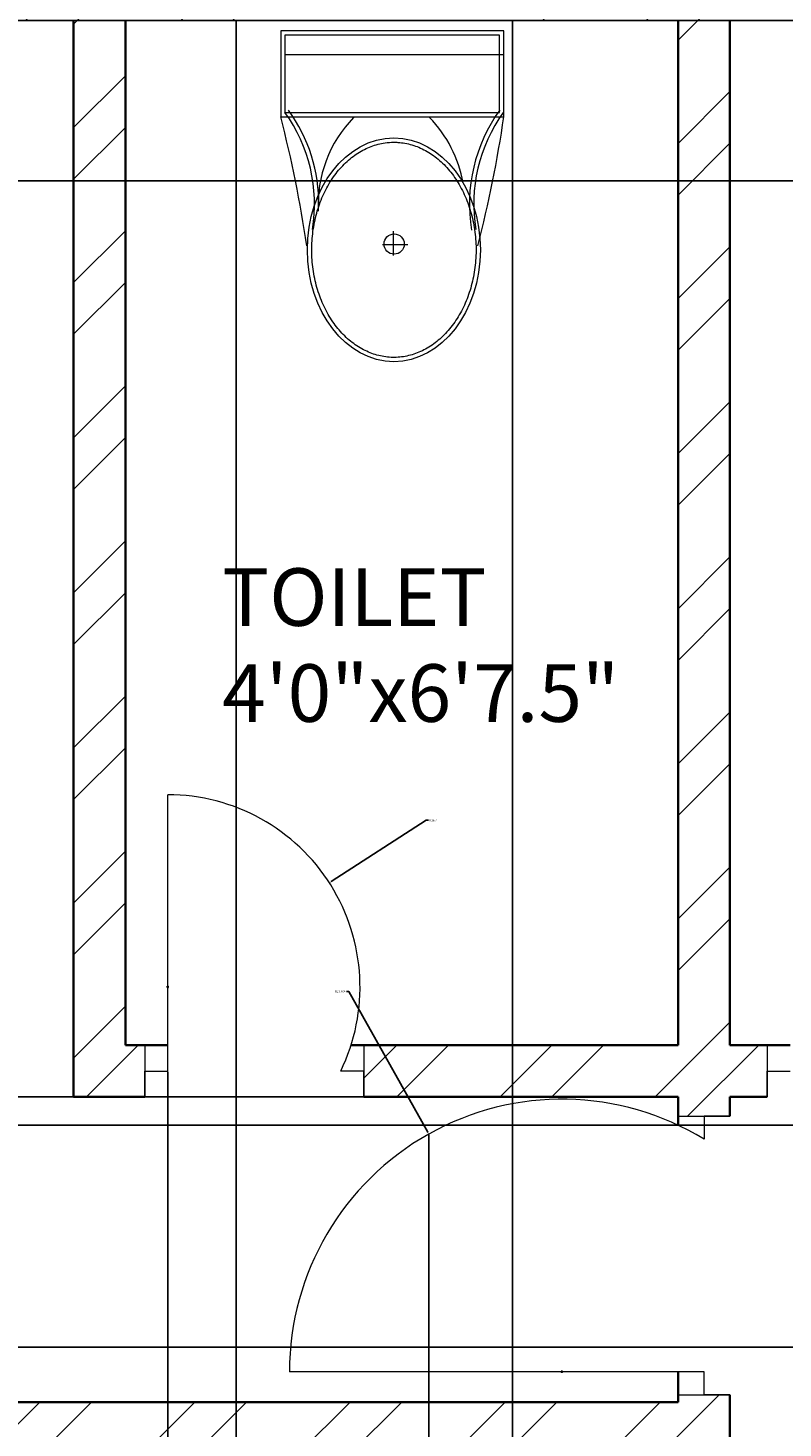
# Model space of a CAD drawing. Units: inches. Extents: x 1748 to 2382, y 1346 to 2284.
# Tile 23 of 26: x 2022 to 2088, y 2102 to 2223. Entities that reach past the tile are written whole.
import ezdxf

# ---------------------------------------------------------------- set-up
doc = ezdxf.new("R2010")
doc.units = ezdxf.units.IN
for name, color, linetype, lineweight in [('A-ANNO-DIMS', 2, 'Continuous', 18), ('A-AREA-IDEN', 7, 'Continuous', 18), ('A-DOOR', 21, 'Continuous', 18), ('A-FLOR-FIXT', 7, 'Continuous', 18), ('A-WALL', 7, 'Continuous', 35), ('A-WALL-PATT', 9, 'Continuous', 13)]:
    doc.layers.add(name, color=color, linetype=linetype, lineweight=lineweight)
doc.styles.get("Standard").update_dxf_attribs({"font": 'arial.ttf'})
doc.dimstyles.get("Standard").update_dxf_attribs({"dimtxt": 0.18, "dimasz": 0.18, "dimexe": 0.18, "dimexo": 0.0625, "dimgap": 0.09, "dimtad": 0, "dimtih": 1, "dimtoh": 1, "dimdec": 4, "dimzin": 0, "dimdsep": 46, "dimtxsty": 'Standard', "dimcen": 0.09, "dimadec": 0, "dimazin": 0, "dimtfac": 1, "dimtdec": 4, "dimtofl": 0, "dimtmove": 0, "dimatfit": 3, "dimfxl": 1, "dimtolj": 1, "dimtzin": 0, "dimarcsym": 0})

# ---------------------------------------------------------------- blocks, each defined once
blk = doc.blocks.new('A$C31115884')
for p, q in [((257.5, 466.4), (257.5, 523.2)), ((283.1, 497.7), (223.4, 497.7)), ((0, 200), (0, 0)), ((520, 200), (0, 200)), ((520, 0), (520, 200)), ((10, 190), (10, 10)), ((510, 190), (10, 190)), ((510, 10), (510, 190)), ((510, 54.5), (0, 54.5)), ((10, 10), (510, 10)), ((0, 0), (520, 0))]:
    blk.add_line(p, q)
blk.add_circle((255.6, 496.4), 23.6)
for centre, radius, start, end in [((2777.7, -204.6), 2807, 165.4549, 171.7133), ((3237, 905), 2807, 188.2867, 194.5451), ((-294.5, 403.3), 364.7, 324.2091, 9.3499), ((-294.5, 403.3), 374.7, 324.2091, 9.3499), ((805.8, 403.3), 364.7, 170.6501, 215.7909), ((139.5, 406.2), 293.5, 315.8436, 2.6563), ((805.8, 403.3), 374.7, 179.2036, 215.7909), ((383.6, 406.2), 293.5, 190.2774, 224.1564)]:
    blk.add_arc(centre, radius, start, end)
blk.add_ellipse((256.2, 509.9), major_axis=(0, -260.7), ratio=0.772727)
blk.add_open_spline([(256.2, 259.2), (263.1, 259.2), (270, 259.7), (287.8, 262.3), (298.7, 265.1), (319.9, 273.1), (330.2, 278.4), (350.1, 291.1), (359.7, 298.7), (377.7, 315.9), (386.2, 325.5), (401.7, 346.6), (408.8, 358.1), (421.3, 382.5), (426.8, 395.5), (435.9, 422.4), (439.5, 436.4), (444.8, 465.1), (446.5, 479.7), (447.9, 509.2), (447.6, 524), (445, 553.3), (442.7, 567.8), (436.3, 596), (432.1, 609.7), (421.9, 636), (416, 648.6), (402.5, 672.1), (395, 683), (378.6, 703), (369.8, 712.1), (351.1, 728), (341.3, 734.8), (320.9, 746.2), (310.4, 750.7), (288.9, 757.3), (278, 759.4), (256, 761), (245, 760.6), (223.1, 757.2), (212.3, 754.3), (191.1, 746.1), (180.8, 740.7), (160.9, 727.8), (151.4, 720.1), (133.5, 702.7), (125.1, 693), (109.6, 671.7), (102.6, 660.2), (90.2, 635.7), (84.9, 622.7), (76, 595.6), (72.4, 581.6), (67.2, 552.9), (65.6, 538.2), (64.4, 508.8), (64.8, 494), (67.5, 464.7), (69.9, 450.2), (76.6, 422), (80.8, 408.3), (91.1, 382.2), (97.2, 369.7), (110.8, 346.3), (118.4, 335.4), (134.8, 315.6), (143.7, 306.7), (162.4, 290.9), (172.3, 284.2), (192.8, 273), (203.3, 268.6), (224.8, 262.2), (235.8, 260.2), (249.9, 259.3), (253, 259.2), (256.2, 259.2)], degree=3, knots=[0, 0, 0, 0, 0.110105, 0.110105, 0.285049, 0.285049, 0.459994, 0.459994, 0.634938, 0.634938, 0.809882, 0.809882, 0.984827, 0.984827, 1.159771, 1.159771, 1.334715, 1.334715, 1.50966, 1.50966, 1.684604, 1.684604, 1.859549, 1.859549, 2.034493, 2.034493, 2.209437, 2.209437, 2.384382, 2.384382, 2.559326, 2.559326, 2.73427, 2.73427, 2.909215, 2.909215, 3.084159, 3.084159, 3.259103, 3.259103, 3.434048, 3.434048, 3.608992, 3.608992, 3.783936, 3.783936, 3.958881, 3.958881, 4.133825, 4.133825, 4.30877, 4.30877, 4.483714, 4.483714, 4.658658, 4.658658, 4.833603, 4.833603, 5.008547, 5.008547, 5.183491, 5.183491, 5.358436, 5.358436, 5.53338, 5.53338, 5.708324, 5.708324, 5.883269, 5.883269, 6.058213, 6.058213, 6.233158, 6.233158, 6.283185, 6.283185, 6.283185, 6.283185])
blk = doc.blocks.new('*D51')
at = {"layer": 'A-ANNO-DIMS', "color": 0, "lineweight": -2, "transparency": 16777216}
for p, q in [((1968.44, 2223.79), (1968.44, 1360.47)), ((2040.07, 2223.79), (2040.07, 1360.47)), ((1968.62, 1360.65), (2003.86, 1360.65)), ((2039.89, 1360.65), (2004.65, 1360.65))]:
    blk.add_line(p, q, dxfattribs=at)
at = {"layer": 'A-ANNO-DIMS', "color": 0, "transparency": 16777216}
for points in [[(1968.62, 1360.68), (1968.62, 1360.62), (1968.44, 1360.65)], [(2039.89, 1360.68), (2039.89, 1360.62), (2040.07, 1360.65)]]:
    blk.add_solid(points, dxfattribs=at)
at = {"layer": 'Defpoints', "color": 0, "transparency": 16777216}
for p in [(1968.44, 2223.85), (2040.07, 2223.85), (2040.07, 1360.65)]:
    blk.add_point(p, dxfattribs=at)
at = {"layer": 'A-ANNO-DIMS', "color": 0, "transparency": 16777216, "insert": (2004.26, 1360.65), "char_height": 0.18, "attachment_point": 5}
blk.add_mtext('\\A1;71.62', dxfattribs=at)
blk = doc.blocks.new('*D52')
at = {"layer": 'A-ANNO-DIMS', "color": 0, "lineweight": -2, "transparency": 16777216}
for p, q in [((2064.07, 2223.79), (2064.07, 1360.47)), ((2091.4, 2223.79), (2091.4, 1360.47)), ((2064.25, 1360.65), (2077.34, 1360.65)), ((2091.22, 1360.65), (2078.13, 1360.65))]:
    blk.add_line(p, q, dxfattribs=at)
at = {"layer": 'A-ANNO-DIMS', "color": 0, "transparency": 16777216}
for points in [[(2064.25, 1360.68), (2064.25, 1360.62), (2064.07, 1360.65)], [(2091.22, 1360.68), (2091.22, 1360.62), (2091.4, 1360.65)]]:
    blk.add_solid(points, dxfattribs=at)
at = {"layer": 'Defpoints', "color": 0, "transparency": 16777216}
for p in [(2064.07, 2223.85), (2091.4, 2223.85), (2091.4, 1360.65)]:
    blk.add_point(p, dxfattribs=at)
at = {"layer": 'A-ANNO-DIMS', "color": 0, "transparency": 16777216, "insert": (2077.73, 1360.65), "char_height": 0.18, "attachment_point": 5}
blk.add_mtext('\\A1;27.33', dxfattribs=at)
blk = doc.blocks.new('*D68')
at = {"layer": 'A-ANNO-DIMS', "color": 0, "lineweight": -2, "transparency": 16777216}
for p, q in [((1865.52, 2223.85), (2339.54, 2223.85)), ((2339.36, 2223.67), (2339.36, 2217.07)), ((2339.36, 2210.1), (2339.36, 2216.7)), ((1865.52, 2209.92), (2339.54, 2209.92))]:
    blk.add_line(p, q, dxfattribs=at)
at = {"layer": 'A-ANNO-DIMS', "color": 0, "transparency": 16777216}
for points in [[(2339.33, 2223.67), (2339.39, 2223.67), (2339.36, 2223.85)], [(2339.33, 2210.1), (2339.39, 2210.1), (2339.36, 2209.92)]]:
    blk.add_solid(points, dxfattribs=at)
at = {"layer": 'Defpoints', "color": 0, "transparency": 16777216}
for p in [(1865.46, 2223.85), (2339.36, 2223.85), (1865.46, 2209.92)]:
    blk.add_point(p, dxfattribs=at)
at = {"layer": 'A-ANNO-DIMS', "color": 0, "transparency": 16777216, "insert": (2339.36, 2216.88), "char_height": 0.18, "attachment_point": 5}
blk.add_mtext('\\A1;13.93', dxfattribs=at)
blk = doc.blocks.new('*D75')
at = {"layer": 'A-ANNO-DIMS', "color": 0, "lineweight": -2, "transparency": 16777216}
for p, q in [((2078.4, 2130.35), (1779.88, 2130.35)), ((1780.06, 2130.17), (1780.06, 2117.28)), ((1780.06, 2104.03), (1780.06, 2116.92)), ((2078.4, 2103.85), (1779.88, 2103.85))]:
    blk.add_line(p, q, dxfattribs=at)
at = {"layer": 'A-ANNO-DIMS', "color": 0, "transparency": 16777216}
for points in [[(1780.03, 2130.17), (1780.09, 2130.17), (1780.06, 2130.35)], [(1780.03, 2104.03), (1780.09, 2104.03), (1780.06, 2103.85)]]:
    blk.add_solid(points, dxfattribs=at)
at = {"layer": 'Defpoints', "color": 0, "transparency": 16777216}
for p in [(1780.06, 2130.35), (2078.46, 2130.35), (2078.46, 2103.85)]:
    blk.add_point(p, dxfattribs=at)
at = {"layer": 'A-ANNO-DIMS', "color": 0, "transparency": 16777216, "insert": (1780.06, 2117.1), "char_height": 0.18, "attachment_point": 5}
blk.add_mtext('\\A1;26.5', dxfattribs=at)
blk = doc.blocks.new('*D77')
at = {"layer": 'A-ANNO-DIMS', "color": 0, "lineweight": -2, "transparency": 16777216}
for p, q in [((1870.02, 2127.89), (2339.54, 2127.89)), ((2339.36, 2127.71), (2339.36, 2118.43)), ((2339.36, 2108.79), (2339.36, 2118.07)), ((1870.02, 2108.61), (2339.54, 2108.61))]:
    blk.add_line(p, q, dxfattribs=at)
at = {"layer": 'A-ANNO-DIMS', "color": 0, "transparency": 16777216}
for points in [[(2339.33, 2127.71), (2339.39, 2127.71), (2339.36, 2127.89)], [(2339.33, 2108.79), (2339.39, 2108.79), (2339.36, 2108.61)]]:
    blk.add_solid(points, dxfattribs=at)
at = {"layer": 'Defpoints', "color": 0, "transparency": 16777216}
for p in [(1869.96, 2127.89), (2339.36, 2127.89), (1869.96, 2108.61)]:
    blk.add_point(p, dxfattribs=at)
at = {"layer": 'A-ANNO-DIMS', "color": 0, "transparency": 16777216, "insert": (2339.36, 2118.25), "char_height": 0.18, "attachment_point": 5}
blk.add_mtext('\\A1;19.288', dxfattribs=at)
blk = doc.blocks.new('*D78')
at = {"layer": 'A-ANNO-DIMS', "color": 0, "lineweight": -2, "transparency": 16777216}
for p, q in [((2034.13, 2132.54), (2034.13, 1360.47)), ((2056.8, 2127.06), (2056.8, 1360.47)), ((2034.31, 1360.65), (2045, 1360.65)), ((2056.62, 1360.65), (2045.93, 1360.65))]:
    blk.add_line(p, q, dxfattribs=at)
at = {"layer": 'A-ANNO-DIMS', "color": 0, "transparency": 16777216}
for points in [[(2034.31, 1360.68), (2034.31, 1360.62), (2034.13, 1360.65)], [(2056.62, 1360.68), (2056.62, 1360.62), (2056.8, 1360.65)]]:
    blk.add_solid(points, dxfattribs=at)
at = {"layer": 'Defpoints', "color": 0, "transparency": 16777216}
for p in [(2034.13, 2132.6), (2056.8, 2127.13), (2056.8, 1360.65)]:
    blk.add_point(p, dxfattribs=at)
at = {"layer": 'A-ANNO-DIMS', "color": 0, "transparency": 16777216, "insert": (2045.47, 1360.65), "char_height": 0.18, "attachment_point": 5}
blk.add_mtext('\\A1;22.663', dxfattribs=at)
blk = doc.blocks.new('*D88')
at = {"layer": 'A-ANNO-DIMS', "color": 0, "lineweight": -2, "transparency": 16777216}
for p, q in [((2049.67, 2139.51), (2049.85, 2139.51)), ((2049.85, 2139.51), (2056.71, 2127.28)), ((2068.28, 2106.49), (2068.46, 2106.49)), ((2068.37, 2106.4), (2068.37, 2106.58))]:
    blk.add_line(p, q, dxfattribs=at)
at = {"layer": 'A-ANNO-DIMS', "color": 0, "transparency": 16777216}
blk.add_solid([(2056.74, 2127.3), (2056.68, 2127.27), (2056.8, 2127.13)], dxfattribs=at)
at = {"layer": 'Defpoints', "color": 0, "transparency": 16777216}
for p in [(2056.8, 2127.13), (2068.37, 2106.49)]:
    blk.add_point(p, dxfattribs=at)
at = {"layer": 'A-ANNO-DIMS', "color": 0, "transparency": 16777216, "insert": (2049.12, 2139.51), "char_height": 0.18, "attachment_point": 5}
blk.add_mtext('\\A1;R23.664', dxfattribs=at)
blk = doc.blocks.new('*D99')
at = {"layer": 'A-ANNO-DIMS', "color": 0, "lineweight": -2, "transparency": 16777216}
for p, q in [((2056.59, 2154.38), (2048.32, 2149.05)), ((2056.77, 2154.38), (2056.59, 2154.38)), ((2034.13, 2139.81), (2034.13, 2139.99)), ((2034.04, 2139.9), (2034.22, 2139.9))]:
    blk.add_line(p, q, dxfattribs=at)
at = {"layer": 'A-ANNO-DIMS', "color": 0, "transparency": 16777216}
blk.add_solid([(2048.31, 2149.07), (2048.34, 2149.02), (2048.17, 2148.95)], dxfattribs=at)
at = {"layer": 'Defpoints', "color": 0, "transparency": 16777216}
for p in [(2048.17, 2148.95), (2034.13, 2139.9)]:
    blk.add_point(p, dxfattribs=at)
at = {"layer": 'A-ANNO-DIMS', "color": 0, "transparency": 16777216, "insert": (2057.18, 2154.38), "char_height": 0.18, "attachment_point": 5}
blk.add_mtext('\\A1;R16.7', dxfattribs=at)

msp = doc.modelspace()

# ---------------------------------------------------------------- hatches: boundary and pattern name
at = {"layer": 'A-WALL-PATT'}
h = msp.add_hatch(dxfattribs=at)
h.set_pattern_fill('ANSI32', color=256)
h.paths.add_polyline_path([(1908.4445, 2232.8497), (1821.9607, 2232.8497), (1821.9607, 2223.8497), (1865.4607, 2223.8497), (1865.4607, 2209.9185), (1869.9607, 2209.9185), (1869.9607, 2223.8497), (1908.4445, 2223.8497), (1908.4445, 2228.3497)])
h.paths.add_polyline_path([(2040.0683, 2232.8497), (1968.4445, 2232.8497), (1968.4445, 2223.8497), (2025.9607, 2223.8497), (2025.9607, 2130.3497), (2032.1341, 2130.3497), (2032.1341, 2132.5997), (2032.1341, 2134.8497), (2030.4607, 2134.8497), (2030.4607, 2223.8497), (2040.0683, 2223.8497)])
h.paths.add_polyline_path([(2091.3969, 2232.8497), (2064.0683, 2232.8497), (2064.0683, 2223.8497), (2078.4607, 2223.8497), (2078.4607, 2134.8497), (2051.1563, 2134.8497), (2051.1563, 2130.3497), (2078.4607, 2130.3497), (2078.4607, 2128.6813), (2082.9607, 2128.6813), (2082.9607, 2130.3497), (2086.1879, 2130.3497), (2086.1879, 2132.5997), (2086.1879, 2134.8497), (2082.9607, 2134.8497), (2082.9607, 2223.8497), (2091.3969, 2223.8497), (2091.3969, 2228.3497)])
h.paths.add_polyline_path([(2167.0164, 2232.8497), (2115.3969, 2232.8497), (2115.3969, 2223.8497), (2130.9607, 2223.8497), (2130.9607, 2134.8497), (2106.9607, 2134.8497), (2106.9607, 2130.3497), (2135.4607, 2130.3497), (2135.4607, 2223.8497), (2167.0164, 2223.8497), (2167.0164, 2228.3497)])
h.paths.add_polyline_path([(1869.9607, 2149.9185), (1865.4607, 2149.9185), (1865.4607, 2127.8942), (1869.9607, 2127.8942)])
h.paths.add_polyline_path([(2082.9607, 2104.4871), (2080.7107, 2104.4871), (2078.4607, 2104.4871), (2078.4607, 2103.8497), (1869.9607, 2103.8497), (1869.9607, 2108.6062), (1867.7107, 2108.6062), (1865.4607, 2108.6062), (1865.4607, 2103.8497), (1821.9607, 2103.8497), (1821.9607, 2099.3497), (1865.4607, 2099.3497), (1865.4607, 2094.7509), (1869.9607, 2094.7509), (1869.9607, 2099.3497), (2025.9607, 2099.3497), (2025.9607, 2096.4326), (2030.4607, 2096.4326), (2030.4607, 2099.3497), (2082.9607, 2099.3497)])
h.paths.add_polyline_path([(1928.9457, 1401.1212), (2176.8693, 1401.1212), (2176.8693, 1438.214), (1928.9457, 1438.214)], flags=9)
h.paths.add_polyline_path([(2122.2668, 2048.1927), (2177.9387, 2048.1927), (2177.9387, 2066.85), (2122.2668, 2066.85)], flags=9)
h.paths.add_polyline_path([(2272.688, 2153.8197), (2272.688, 2216.746), (2262.3845, 2216.746), (2262.3845, 2153.8197)], flags=9)
h.paths.add_polyline_path([(2157.2928, 2166.5593), (2196.3822, 2166.5593), (2196.3822, 2185.2167), (2157.2928, 2185.2167)], flags=9)
h.paths.add_polyline_path([(2089.3407, 2162.0698), (2124.3987, 2162.0698), (2124.3987, 2180.7272), (2089.3407, 2180.7272)], flags=9)
h.paths.add_polyline_path([(2037.4521, 2160.0913), (2072.5101, 2160.0913), (2072.5101, 2178.7486), (2037.4521, 2178.7486)], flags=9)
h.paths.add_polyline_path([(1884.7894, 2104.1554), (1923.6297, 2104.1554), (1923.6297, 2122.8127), (1884.7894, 2122.8127)], flags=9)
h.paths.add_polyline_path([(1851.2832, 2142.9749), (1851.2832, 2199.3051), (1840.9796, 2199.3051), (1840.9796, 2142.9749)], flags=9)
h.paths.add_polyline_path([(1844.8763, 2017.2834), (1844.8763, 2073.6136), (1834.5728, 2073.6136), (1834.5728, 2017.2834)], flags=9)
h.paths.add_polyline_path([(1897.1577, 2073.1279), (1935.9981, 2073.1279), (1935.9981, 2091.7853), (1897.1577, 2091.7853)], flags=9)
h.paths.add_polyline_path([(1952.3395, 1802.4231), (2008.0114, 1802.4231), (2008.0114, 1821.0805), (1952.3395, 1821.0805)], flags=9)
h.paths.add_polyline_path([(1978.8184, 1857.6841), (2017.7338, 1857.6841), (2017.7338, 1876.3415), (1978.8184, 1876.3415)], flags=9)
h.paths.add_polyline_path([(1979.6513, 1925.9516), (2008.8089, 1925.9516), (2008.8089, 1944.6089), (1979.6513, 1944.6089)], flags=9)
h.paths.add_polyline_path([(1838.5553, 1860.3527), (1877.3957, 1860.3527), (1877.3957, 1879.01), (1838.5553, 1879.01)], flags=9)
h.paths.add_polyline_path([(1883.9018, 1787.3013), (1883.9018, 1843.6315), (1873.5983, 1843.6315), (1873.5983, 1787.3013)], flags=9)
h.paths.add_polyline_path([(1873.7079, 1509.1938), (1873.7079, 1583.7709), (1863.4044, 1583.7709), (1863.4044, 1509.1938)], flags=9)
h.paths.add_polyline_path([(1916.2259, 1603.3681), (1955.0663, 1603.3681), (1955.0663, 1622.0254), (1916.2259, 1622.0254)], flags=9)
h.paths.add_polyline_path([(1876.3013, 1636.757), (1876.3013, 1693.0871), (1865.9978, 1693.0871), (1865.9978, 1636.757)], flags=9)
h.paths.add_polyline_path([(1921.3138, 1521.8316), (1964.0662, 1521.8316), (1964.0662, 1540.489), (1921.3138, 1540.489)], flags=9)
h.paths.add_polyline_path([(2017.5657, 1497.5078), (2046.7983, 1497.5078), (2046.7983, 1516.1651), (2017.5657, 1516.1651)], flags=9)
h.paths.add_polyline_path([(2066.8661, 1499.3902), (2096.0988, 1499.3902), (2096.0988, 1518.0475), (2066.8661, 1518.0475)], flags=9)
h.paths.add_polyline_path([(2155.4835, 1571.6596), (2198.2358, 1571.6596), (2198.2358, 1590.3169), (2155.4835, 1590.3169)], flags=9)
h.paths.add_polyline_path([(2094.9136, 1664.6812), (2150.5855, 1664.6812), (2150.5855, 1683.3386), (2094.9136, 1683.3386)], flags=9)
h.paths.add_polyline_path([(2257.6902, 1863.1628), (2269.8935, 1863.1628), (2269.8935, 1873.4664), (2257.6902, 1873.4664)], flags=9)
h.paths.add_polyline_path([(2164.0748, 1880.3089), (2189.8694, 1880.3089), (2189.8694, 1890.6124), (2164.0748, 1890.6124)], flags=9)
h.paths.add_polyline_path([(2239.4394, 1931.0585), (2268.8187, 1931.0585), (2268.8187, 1949.7159), (2239.4394, 1949.7159)], flags=9)
h = msp.add_hatch(dxfattribs=at)
h.set_pattern_fill('ANSI32', color=256)
h.paths.add_polyline_path([(2297.4607, 2232.8497), (2203.0164, 2232.8497), (2203.0164, 2223.8497), (2244.9607, 2223.8497), (2244.9607, 2127.8554), (2249.4607, 2127.8554), (2249.4607, 2223.8497), (2297.4607, 2223.8497)])
h.paths.add_polyline_path([(2297.4607, 2103.8497), (2249.4607, 2103.8497), (2249.4607, 2106.7497), (2247.2107, 2106.7497), (2244.9607, 2106.7497), (2244.9607, 2103.8497), (2130.9607, 2103.8497), (2130.9607, 2099.3497), (2288.4607, 2099.3497), (2288.4607, 2077.2008), (2297.4607, 2077.2008)])
h.paths.add_polyline_path([(1928.9457, 1401.1212), (2176.8693, 1401.1212), (2176.8693, 1438.214), (1928.9457, 1438.214)], flags=9)
h.paths.add_polyline_path([(2122.2668, 2048.1927), (2177.9387, 2048.1927), (2177.9387, 2066.85), (2122.2668, 2066.85)], flags=9)
h.paths.add_polyline_path([(2272.688, 2153.8197), (2272.688, 2216.746), (2262.3845, 2216.746), (2262.3845, 2153.8197)], flags=25)
h.paths.add_polyline_path([(2157.2928, 2166.5593), (2196.3822, 2166.5593), (2196.3822, 2185.2167), (2157.2928, 2185.2167)], flags=9)
h.paths.add_polyline_path([(2089.3407, 2162.0698), (2124.3987, 2162.0698), (2124.3987, 2180.7272), (2089.3407, 2180.7272)], flags=9)
h.paths.add_polyline_path([(2037.4521, 2160.0913), (2072.5101, 2160.0913), (2072.5101, 2178.7486), (2037.4521, 2178.7486)], flags=9)
h.paths.add_polyline_path([(1884.7894, 2104.1554), (1923.6297, 2104.1554), (1923.6297, 2122.8127), (1884.7894, 2122.8127)], flags=9)
h.paths.add_polyline_path([(1851.2832, 2142.9749), (1851.2832, 2199.3051), (1840.9796, 2199.3051), (1840.9796, 2142.9749)], flags=9)
h.paths.add_polyline_path([(1844.8763, 2017.2834), (1844.8763, 2073.6136), (1834.5728, 2073.6136), (1834.5728, 2017.2834)], flags=9)
h.paths.add_polyline_path([(1897.1577, 2073.1279), (1935.9981, 2073.1279), (1935.9981, 2091.7853), (1897.1577, 2091.7853)], flags=9)
h.paths.add_polyline_path([(1952.3395, 1802.4231), (2008.0114, 1802.4231), (2008.0114, 1821.0805), (1952.3395, 1821.0805)], flags=9)
h.paths.add_polyline_path([(1978.8184, 1857.6841), (2017.7338, 1857.6841), (2017.7338, 1876.3415), (1978.8184, 1876.3415)], flags=9)
h.paths.add_polyline_path([(1979.6513, 1925.9516), (2008.8089, 1925.9516), (2008.8089, 1944.6089), (1979.6513, 1944.6089)], flags=9)
h.paths.add_polyline_path([(1838.5553, 1860.3527), (1877.3957, 1860.3527), (1877.3957, 1879.01), (1838.5553, 1879.01)], flags=9)
h.paths.add_polyline_path([(1883.9018, 1787.3013), (1883.9018, 1843.6315), (1873.5983, 1843.6315), (1873.5983, 1787.3013)], flags=9)
h.paths.add_polyline_path([(1873.7079, 1509.1938), (1873.7079, 1583.7709), (1863.4044, 1583.7709), (1863.4044, 1509.1938)], flags=9)
h.paths.add_polyline_path([(1916.2259, 1603.3681), (1955.0663, 1603.3681), (1955.0663, 1622.0254), (1916.2259, 1622.0254)], flags=9)
h.paths.add_polyline_path([(1876.3013, 1636.757), (1876.3013, 1693.0871), (1865.9978, 1693.0871), (1865.9978, 1636.757)], flags=9)
h.paths.add_polyline_path([(1921.3138, 1521.8316), (1964.0662, 1521.8316), (1964.0662, 1540.489), (1921.3138, 1540.489)], flags=9)
h.paths.add_polyline_path([(2017.5657, 1497.5078), (2046.7983, 1497.5078), (2046.7983, 1516.1651), (2017.5657, 1516.1651)], flags=9)
h.paths.add_polyline_path([(2066.8661, 1499.3902), (2096.0988, 1499.3902), (2096.0988, 1518.0475), (2066.8661, 1518.0475)], flags=9)
h.paths.add_polyline_path([(2155.4835, 1571.6596), (2198.2358, 1571.6596), (2198.2358, 1590.3169), (2155.4835, 1590.3169)], flags=9)
h.paths.add_polyline_path([(2094.9136, 1664.6812), (2150.5855, 1664.6812), (2150.5855, 1683.3386), (2094.9136, 1683.3386)], flags=9)
h.paths.add_polyline_path([(2257.6902, 1863.1628), (2269.8935, 1863.1628), (2269.8935, 1873.4664), (2257.6902, 1873.4664)], flags=9)
h.paths.add_polyline_path([(2164.0748, 1880.3089), (2189.8694, 1880.3089), (2189.8694, 1890.6124), (2164.0748, 1890.6124)], flags=9)
h.paths.add_polyline_path([(2239.4394, 1931.0585), (2268.8187, 1931.0585), (2268.8187, 1949.7159), (2239.4394, 1949.7159)], flags=9)
h = msp.add_hatch(dxfattribs=at)
h.set_pattern_fill('ANSI32', color=256)
h.paths.add_polyline_path([(1919.6777, 1476.8497), (1900.6426, 1476.8497), (1900.6426, 1522.0826), (1898.3926, 1522.0826), (1896.1426, 1522.0826), (1896.1426, 1476.8497), (1857.1426, 1476.8497), (1857.1426, 1467.8497), (1896.1426, 1467.8497), (1919.6777, 1467.8497), (1919.6777, 1472.3497)])
h.paths.add_polyline_path([(2018.7873, 1472.3497), (2018.7873, 1476.8497), (2010.9607, 1476.8497), (2010.9607, 1560.8497), (2034.9607, 1560.8497), (2034.9607, 1565.3497), (2006.4607, 1565.3497), (2006.4607, 1476.8497), (1955.6777, 1476.8497), (1955.6777, 1467.8497), (2018.7873, 1467.8497)])
h.paths.add_polyline_path([(2152.3354, 1472.3497), (2152.3354, 1476.8497), (2115.9607, 1476.8497), (2115.9607, 1565.3497), (2109.2204, 1565.3497), (2109.2204, 1563.0997), (2109.2204, 1560.8497), (2111.4607, 1560.8497), (2111.4607, 1476.8497), (2095.3617, 1476.8497), (2095.3617, 1467.8497), (2152.3354, 1467.8497)])
h.paths.add_polyline_path([(2071.3617, 1476.8497), (2063.4607, 1476.8497), (2063.4607, 1560.8497), (2090.1865, 1560.8497), (2090.1865, 1565.3497), (2063.4607, 1565.3497), (2063.4607, 1572.5485), (2061.2107, 1572.5485), (2058.9607, 1572.5485), (2058.9607, 1565.3497), (2055.6281, 1565.3497), (2055.6281, 1560.8497), (2058.9607, 1560.8497), (2058.9607, 1476.8497), (2042.7873, 1476.8497), (2042.7873, 1467.8497), (2071.3617, 1467.8497), (2071.3617, 1472.3497)])
h.paths.add_polyline_path([(2297.4607, 1506.5652), (2288.4607, 1506.5652), (2288.4607, 1476.8497), (2212.3354, 1476.8497), (2212.3354, 1467.8497), (2297.4607, 1467.8497)])
h.paths.add_polyline_path([(2297.4607, 1645.3038), (2288.4607, 1645.3038), (2288.4607, 1605.8497), (2058.9607, 1605.8497), (2058.9607, 1600.1857), (2061.2107, 1600.1857), (2063.4607, 1600.1857), (2063.4607, 1601.3497), (2288.4607, 1601.3497), (2288.4607, 1566.5652), (2297.4607, 1566.5652)])
h.paths.add_polyline_path([(2010.9607, 1609.0561), (2008.7107, 1609.0561), (2006.4607, 1609.0561), (2006.4607, 1605.8497), (1900.6426, 1605.8497), (1900.6426, 1609.7171), (1898.3926, 1609.7171), (1896.1426, 1609.7171), (1896.1426, 1605.8497), (1857.1426, 1605.8497), (1857.1426, 1601.3497), (1896.1426, 1601.3497), (1896.1426, 1542.5447), (1900.6426, 1542.5447), (1900.6426, 1601.3497), (2010.9607, 1601.3497)])
h.paths.add_polyline_path([(1928.9457, 1401.1212), (2176.8693, 1401.1212), (2176.8693, 1438.214), (1928.9457, 1438.214)], flags=9)
h.paths.add_polyline_path([(2122.2668, 2048.1927), (2177.9387, 2048.1927), (2177.9387, 2066.85), (2122.2668, 2066.85)], flags=9)
h.paths.add_polyline_path([(2272.688, 2153.8197), (2272.688, 2216.746), (2262.3845, 2216.746), (2262.3845, 2153.8197)], flags=9)
h.paths.add_polyline_path([(2157.2928, 2166.5593), (2196.3822, 2166.5593), (2196.3822, 2185.2167), (2157.2928, 2185.2167)], flags=9)
h.paths.add_polyline_path([(2089.3407, 2162.0698), (2124.3987, 2162.0698), (2124.3987, 2180.7272), (2089.3407, 2180.7272)], flags=9)
h.paths.add_polyline_path([(2037.4521, 2160.0913), (2072.5101, 2160.0913), (2072.5101, 2178.7486), (2037.4521, 2178.7486)], flags=9)
h.paths.add_polyline_path([(1884.7894, 2104.1554), (1923.6297, 2104.1554), (1923.6297, 2122.8127), (1884.7894, 2122.8127)], flags=9)
h.paths.add_polyline_path([(1851.2832, 2142.9749), (1851.2832, 2199.3051), (1840.9796, 2199.3051), (1840.9796, 2142.9749)], flags=9)
h.paths.add_polyline_path([(1844.8763, 2017.2834), (1844.8763, 2073.6136), (1834.5728, 2073.6136), (1834.5728, 2017.2834)], flags=9)
h.paths.add_polyline_path([(1897.1577, 2073.1279), (1935.9981, 2073.1279), (1935.9981, 2091.7853), (1897.1577, 2091.7853)], flags=9)
h.paths.add_polyline_path([(1952.3395, 1802.4231), (2008.0114, 1802.4231), (2008.0114, 1821.0805), (1952.3395, 1821.0805)], flags=9)
h.paths.add_polyline_path([(1978.8184, 1857.6841), (2017.7338, 1857.6841), (2017.7338, 1876.3415), (1978.8184, 1876.3415)], flags=9)
h.paths.add_polyline_path([(1979.6513, 1925.9516), (2008.8089, 1925.9516), (2008.8089, 1944.6089), (1979.6513, 1944.6089)], flags=9)
h.paths.add_polyline_path([(1838.5553, 1860.3527), (1877.3957, 1860.3527), (1877.3957, 1879.01), (1838.5553, 1879.01)], flags=9)
h.paths.add_polyline_path([(1883.9018, 1787.3013), (1883.9018, 1843.6315), (1873.5983, 1843.6315), (1873.5983, 1787.3013)], flags=9)
h.paths.add_polyline_path([(1873.7079, 1509.1938), (1873.7079, 1583.7709), (1863.4044, 1583.7709), (1863.4044, 1509.1938)], flags=9)
h.paths.add_polyline_path([(1916.2259, 1603.3681), (1955.0663, 1603.3681), (1955.0663, 1622.0254), (1916.2259, 1622.0254)], flags=9)
h.paths.add_polyline_path([(1876.3013, 1636.757), (1876.3013, 1693.0871), (1865.9978, 1693.0871), (1865.9978, 1636.757)], flags=9)
h.paths.add_polyline_path([(1921.3138, 1521.8316), (1964.0662, 1521.8316), (1964.0662, 1540.489), (1921.3138, 1540.489)], flags=9)
h.paths.add_polyline_path([(2017.5657, 1497.5078), (2046.7983, 1497.5078), (2046.7983, 1516.1651), (2017.5657, 1516.1651)], flags=9)
h.paths.add_polyline_path([(2066.8661, 1499.3902), (2096.0988, 1499.3902), (2096.0988, 1518.0475), (2066.8661, 1518.0475)], flags=9)
h.paths.add_polyline_path([(2155.4835, 1571.6596), (2198.2358, 1571.6596), (2198.2358, 1590.3169), (2155.4835, 1590.3169)], flags=25)
h.paths.add_polyline_path([(2094.9136, 1664.6812), (2150.5855, 1664.6812), (2150.5855, 1683.3386), (2094.9136, 1683.3386)], flags=9)
h.paths.add_polyline_path([(2257.6902, 1863.1628), (2269.8935, 1863.1628), (2269.8935, 1873.4664), (2257.6902, 1873.4664)], flags=9)
h.paths.add_polyline_path([(2164.0748, 1880.3089), (2189.8694, 1880.3089), (2189.8694, 1890.6124), (2164.0748, 1890.6124)], flags=9)
h.paths.add_polyline_path([(2239.4394, 1931.0585), (2268.8187, 1931.0585), (2268.8187, 1949.7159), (2239.4394, 1949.7159)], flags=9)

# ---------------------------------------------------------------- linework, layer by layer
at = {"layer": 'A-DOOR'}
for p, q in [((2034.1341, 2132.5997), (2034.1341, 2156.5997)), ((2032.1341, 2134.8497), (2032.1341, 2130.3497)), ((2051.1563, 2134.8497), (2051.1563, 2130.3497)), ((2086.1879, 2134.8497), (2086.1879, 2130.3497)), ((2032.1341, 2130.3497), (2032.1341, 2132.5997)), ((2032.1341, 2132.5997), (2034.1341, 2132.5997)), ((2051.1563, 2132.5997), (2049.1563, 2132.5997)), ((2051.1563, 2130.3497), (2051.1563, 2132.5997)), ((2086.1879, 2130.3497), (2086.1879, 2132.5997)), ((2086.1879, 2132.5997), (2088.1879, 2132.5997)), ((2078.4607, 2128.6813), (2082.9607, 2128.6813)), ((2082.9607, 2128.6813), (2080.7107, 2128.6813)), ((2080.7107, 2128.6813), (2080.7107, 2126.6813)), ((2080.7107, 2106.4871), (2044.7107, 2106.4871)), ((2080.7107, 2104.4871), (2080.7107, 2106.4871)), ((2078.4607, 2104.4871), (2082.9607, 2104.4871)), ((2082.9607, 2104.4871), (2080.7107, 2104.4871))]:
    msp.add_line(p, q, dxfattribs=at)
for centre, radius, start, end in [((2034.1341, 2139.8983), 16.7014, 334.086885, 90), ((2068.3747, 2106.4871), 23.664, 58.580681, 180)]:
    msp.add_arc(centre, radius, start, end, dxfattribs=at)
at = {"layer": 'A-WALL'}
for p, q in [((2025.9607, 2223.8497), (2025.9607, 2130.3497)), ((2030.4607, 2223.8497), (2030.4607, 2134.8497)), ((2078.4607, 2223.8497), (2078.4607, 2134.8497)), ((2082.9607, 2223.8497), (2082.9607, 2134.8497)), ((2030.4607, 2134.8497), (2034.1341, 2134.8497)), ((2050.0542, 2134.8497), (2078.4607, 2134.8497)), ((2082.9607, 2134.8497), (2088.1879, 2134.8497)), ((2025.9607, 2130.3497), (2032.1341, 2130.3497)), ((2051.1563, 2130.3497), (2078.4607, 2130.3497)), ((2078.4607, 2130.3497), (2078.4607, 2127.894)), ((2082.9607, 2130.3497), (2086.1879, 2130.3497)), ((2082.9607, 2130.3497), (2082.9607, 2128.6813)), ((2078.4607, 2106.4871), (2078.4607, 2103.8497)), ((1869.9607, 2103.8497), (2078.4607, 2103.8497)), ((2082.9607, 2104.4871), (2082.9607, 2099.3497))]:
    msp.add_line(p, q, dxfattribs=at)

# ---------------------------------------------------------------- block references
at = {"layer": 'A-FLOR-FIXT', "xscale": 0.0372717239612423, "yscale": 0.0372717239612423, "zscale": 0.0372717239612423, "rotation": 180}
msp.add_blockref('A$C31115884', (2063.3244, 2222.9281), dxfattribs=at)

# ---------------------------------------------------------------- texts
at = {"layer": 'A-AREA-IDEN', "insert": (2038.8659, 2176.264), "char_height": 5, "attachment_point": 1}
msp.add_mtext_dynamic_manual_height_columns('TOILET\\P4\'0"x6\'7.5"', width=134.841065, gutter_width=12.5, heights=[0], dxfattribs=at)

# ---------------------------------------------------------------- dimensions: what is measured, and where the dimension line sits
at = {"layer": 'A-ANNO-DIMS'}
for base, p1, p2, override, picture, middle in [((2339.3607, 2223.8497), (1865.4607, 2209.9185), (1865.4607, 2223.8497), {"dimdec": 2, "dimlfac": 1, "dimrnd": 0, "dimzin": 0, "dimdsep": 46, "dimlunit": 2}, '*D68', (2339.3607, 2216.8841)), ((1780.0607, 2130.3497), (2078.4607, 2103.8497), (2078.4607, 2130.3497), {"dimdec": 1, "dimlfac": 1, "dimrnd": 0, "dimzin": 0, "dimdsep": 46, "dimlunit": 2}, '*D75', (1780.0607, 2117.0997)), ((2339.3607, 2127.8942), (1869.9607, 2108.6062), (1869.9607, 2127.8942), {"dimdec": 3, "dimlfac": 1, "dimrnd": 0, "dimzin": 0, "dimdsep": 46, "dimlunit": 2}, '*D77', (2339.3607, 2118.2502))]:
    dim = msp.add_linear_dim(base=base, p1=p1, p2=p2, angle=90, dimstyle='Standard', override=override, dxfattribs=at)
    dim.commit()
    dim.dimension.update_dxf_attribs({"geometry": picture, "text_midpoint": middle})
for base, p1, p2, override, picture, middle in [((2040.0683, 1360.6451), (1968.4445, 2223.8497), (2040.0683, 2223.8497), {"dimdec": 2, "dimlfac": 1, "dimrnd": 0, "dimzin": 0, "dimdsep": 46, "dimlunit": 2}, '*D51', (2004.2564, 1360.6451)), ((2091.3969, 1360.6451), (2064.0683, 2223.8497), (2091.3969, 2223.8497), {"dimdec": 2, "dimlfac": 1, "dimrnd": 0, "dimzin": 0, "dimdsep": 46, "dimlunit": 2}, '*D52', (2077.7326, 1360.6451)), ((2056.7974, 1360.6451), (2034.1341, 2132.5997), (2056.7974, 2127.1257), {"dimdec": 3, "dimlfac": 1, "dimrnd": 0, "dimzin": 0, "dimdsep": 46, "dimlunit": 2}, '*D78', (2045.4658, 1360.6451))]:
    dim = msp.add_linear_dim(base=base, p1=p1, p2=p2, dimstyle='Standard', override=override, dxfattribs=at)
    dim.commit()
    dim.dimension.update_dxf_attribs({"geometry": picture, "text_midpoint": middle})
for center, mpoint, override, picture, middle in [((2034.1341, 2139.8983), (2048.1704, 2148.9492), {"dimdec": 1, "dimlfac": 1, "dimrnd": 0, "dimzin": 0, "dimdsep": 46, "dimlunit": 2}, '*D99', (2057.1821, 2154.3797)), ((2068.3747, 2106.4871), (2056.7972, 2127.1256), {"dimdec": 3, "dimlfac": 1, "dimrnd": 0, "dimzin": 0, "dimdsep": 46, "dimlunit": 2}, '*D88', (2049.1214, 2139.5087))]:
    dim = msp.add_radius_dim(center=center, mpoint=mpoint, dimstyle='Standard', override=override, dxfattribs=at)
    dim.commit()
    dim.dimension.update_dxf_attribs({"geometry": picture, "text_midpoint": middle, "dimtype": 164})

doc.saveas('drawing.dxf')
